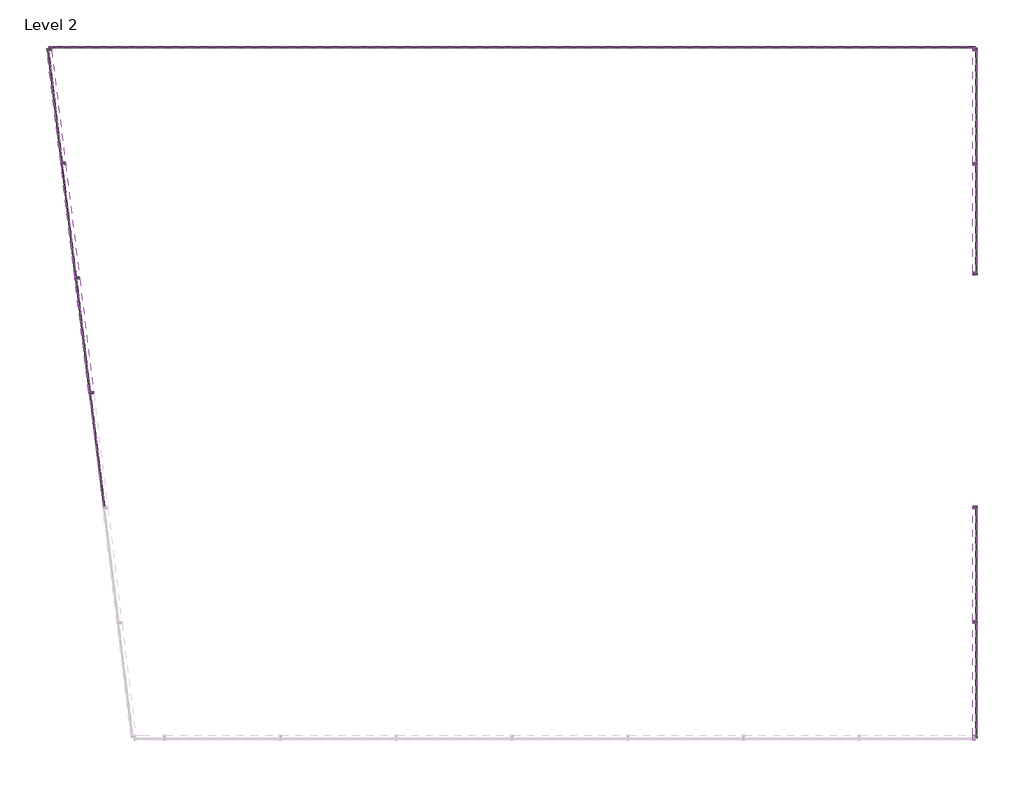
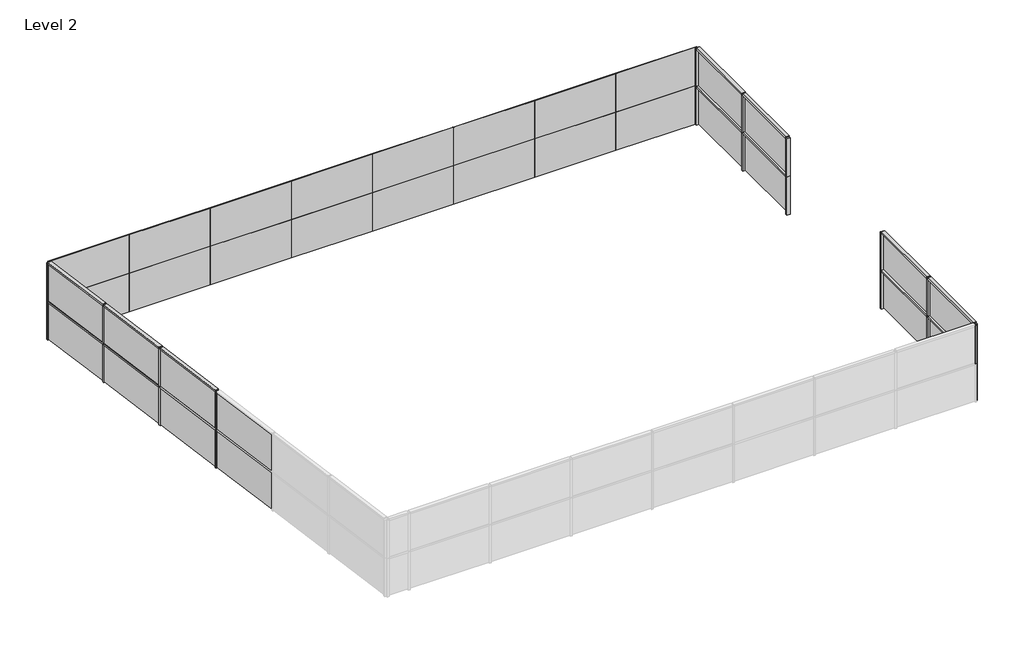
# One storey, part 2 of 2: 35 members, 32 plates.
"""IFC4 building model written with IfcOpenShell, lengths in millimetres."""

from ifc_helpers import new_model, si_unit, origin, place, context, project, spatial, transform, mapped, element, save
from components import member_19d0a4ec, member_8cef0660, member_82905deb, member_4491d118, member_46bdb8c2, system_panel_glazed_1e57f9bb, system_panel_glazed_e46d4b42, system_panel_glazed_2a6c68b7, system_panel_glazed_d483336f

model = new_model("IFC4")

# Units and contexts
model_context = context("Model", 3, world=origin())
ifc_project = project(units=[si_unit("LENGTHUNIT", "METRE", prefix="MILLI")], contexts=[model_context])

# Site, building, storey
site = spatial("IfcSite", under=ifc_project)
building = spatial("IfcBuilding", under=site)
storey = spatial("IfcBuildingStorey", under=building, Name="Level 2", Elevation=3048.0)

# Members
placement = place(None, origin())
member_shape = member_19d0a4ec(model_context)
element("IfcMember", 1, ObjectType="Rectangular Mullion : 2.5\" x 5\" rectangular", at=placement, inside=storey, context=model_context, shape_type="MappedRepresentation", body=[
    mapped(member_shape, transform((-10113.8959567, 8178.7803212, 4572.0), x_axis=(0.0, 0.0, 1.0), y_axis=(-0.9925461516413222, -0.12186934340514595, 0.0), z_axis=(0.12186934340514594, -0.9925461516413221, 0.0))),
])
element("IfcMember", 2, ObjectType="Rectangular Mullion : 2.5\" x 5\" rectangular", at=placement, inside=storey, context=model_context, shape_type="MappedRepresentation", body=[
    mapped(member_shape, transform((-10113.8959567, 8178.7803212, 6096.0), x_axis=(0.0, 0.0, 1.0), y_axis=(-0.9925461516413222, -0.12186934340514603, 0.0), z_axis=(0.12186934340514602, -0.9925461516413221, 0.0))),
])
element("IfcMember", 3, ObjectType="Rectangular Mullion : 2.5\" x 5\" rectangular", at=placement, inside=storey, context=model_context, shape_type="MappedRepresentation", body=[
    mapped(member_shape, transform((13902.5156363, 11109.0476508, 4572.0), x_axis=(0.0, 0.0, 1.0), y_axis=(1.0, 0.0, 0.0), z_axis=(0.0, 1.0, 0.0))),
])
element("IfcMember", 4, ObjectType="Rectangular Mullion : 2.5\" x 5\" rectangular", at=placement, inside=storey, context=model_context, shape_type="MappedRepresentation", body=[
    mapped(member_shape, transform((13902.5156363, 11109.0476508, 6096.0), x_axis=(0.0, 0.0, 1.0), y_axis=(1.0, 0.0, 0.0), z_axis=(0.0, 1.0, 0.0))),
])
element("IfcMember", 5, ObjectType="Rectangular Mullion : 2.5\" x 5\" rectangular", at=placement, inside=storey, context=model_context, shape_type="MappedRepresentation", body=[
    mapped(member_shape, transform((13902.5156363, -946.6363705, 4572.0), x_axis=(0.0, 0.0, 1.0), y_axis=(1.0, 0.0, 0.0), z_axis=(0.0, 1.0, 0.0))),
])
element("IfcMember", 6, ObjectType="Rectangular Mullion : 2.5\" x 5\" rectangular", at=placement, inside=storey, context=model_context, shape_type="MappedRepresentation", body=[
    mapped(member_shape, transform((13902.5156363, -3962.8863708, 4572.0), x_axis=(0.0, 0.0, 1.0), y_axis=(1.0, 0.0, 0.0), z_axis=(0.0, 1.0, 0.0))),
])
element("IfcMember", 7, ObjectType="Rectangular Mullion : 2.5\" x 5\" rectangular", at=placement, inside=storey, context=model_context, shape_type="MappedRepresentation", body=[
    mapped(member_shape, transform((13902.5156363, -946.6363705, 6096.0), x_axis=(0.0, 0.0, 1.0), y_axis=(1.0, 0.0, 0.0), z_axis=(0.0, 1.0, 0.0))),
])
element("IfcMember", 8, ObjectType="Rectangular Mullion : 2.5\" x 5\" rectangular", at=placement, inside=storey, context=model_context, shape_type="MappedRepresentation", body=[
    mapped(member_shape, transform((13902.5156363, -3962.8863708, 6096.0), x_axis=(0.0, 0.0, 1.0), y_axis=(1.0, 0.0, 0.0), z_axis=(0.0, 1.0, 0.0))),
])
member_2_shape = member_8cef0660(model_context)
element("IfcMember", 9, ObjectType="Rectangular Mullion : 2.5\" x 5\" rectangular", at=placement, inside=storey, context=model_context, shape_type="MappedRepresentation", body=[
    mapped(member_2_shape, transform((-9370.9804393, 2128.2189808, 4572.0), x_axis=(0.0, 0.0, 1.0), y_axis=(-0.9925461516413223, -0.12186934340514563, 0.0), z_axis=(0.12186934340514562, -0.9925461516413222, 0.0))),
])
element("IfcMember", 10, ObjectType="Rectangular Mullion : 2.5\" x 5\" rectangular", at=placement, inside=storey, context=model_context, shape_type="MappedRepresentation", body=[
    mapped(member_2_shape, transform((-9742.438198, 5153.499651, 4572.0), x_axis=(0.0, 0.0, 1.0), y_axis=(-0.9925461516413222, -0.12186934340514596, 0.0), z_axis=(0.12186934340514596, -0.9925461516413222, 0.0))),
])
element("IfcMember", 11, ObjectType="Rectangular Mullion : 2.5\" x 5\" rectangular", at=placement, inside=storey, context=model_context, shape_type="MappedRepresentation", body=[
    mapped(member_2_shape, transform((-9370.9804393, 2128.2189808, 6096.0), x_axis=(0.0, 0.0, 1.0), y_axis=(-0.9925461516413223, -0.12186934340514563, 0.0), z_axis=(0.12186934340514562, -0.9925461516413222, 0.0))),
])
element("IfcMember", 12, ObjectType="Rectangular Mullion : 2.5\" x 5\" rectangular", at=placement, inside=storey, context=model_context, shape_type="MappedRepresentation", body=[
    mapped(member_2_shape, transform((-9742.438198, 5153.499651, 6096.0), x_axis=(0.0, 0.0, 1.0), y_axis=(-0.9925461516413222, -0.12186934340514596, 0.0), z_axis=(0.12186934340514596, -0.9925461516413222, 0.0))),
])
member_3_shape = member_82905deb(model_context)
element("IfcMember", 13, ObjectType="Rectangular Mullion : 2.5\" x 5\" rectangular", at=placement, inside=storey, context=model_context, shape_type="MappedRepresentation", body=[
    mapped(member_3_shape, transform((-9367.1110876, 2096.7056405, 4572.0), x_axis=(-0.12186934340514591, 0.9925461516413222, 0.0), y_axis=(-0.9925461516413222, -0.12186934340514591, 0.0), z_axis=(0.0, 0.0, 1.0))),
])
element("IfcMember", 14, ObjectType="Rectangular Mullion : 2.5\" x 5\" rectangular", at=placement, inside=storey, context=model_context, shape_type="MappedRepresentation", body=[
    mapped(member_3_shape, transform((-9367.1110876, 2096.7056405, 6096.0), x_axis=(-0.12186934340514591, 0.9925461516413222, 0.0), y_axis=(-0.9925461516413222, -0.12186934340514591, 0.0), z_axis=(0.0, 0.0, 1.0))),
])
element("IfcMember", 15, ObjectType="Rectangular Mullion : 2.5\" x 5\" rectangular", at=placement, inside=storey, context=model_context, shape_type="MappedRepresentation", body=[
    mapped(member_3_shape, transform((-9738.5688463, 5121.9863107, 4572.0), x_axis=(-0.12186934340514591, 0.9925461516413222, 0.0), y_axis=(-0.9925461516413222, -0.12186934340514591, 0.0), z_axis=(0.0, 0.0, 1.0))),
])
element("IfcMember", 16, ObjectType="Rectangular Mullion : 2.5\" x 5\" rectangular", at=placement, inside=storey, context=model_context, shape_type="MappedRepresentation", body=[
    mapped(member_3_shape, transform((-9738.5688463, 5121.9863107, 6096.0), x_axis=(-0.12186934340514591, 0.9925461516413222, 0.0), y_axis=(-0.9925461516413222, -0.12186934340514591, 0.0), z_axis=(0.0, 0.0, 1.0))),
])
element("IfcMember", 17, ObjectType="Rectangular Mullion : 2.5\" x 5\" rectangular", at=placement, inside=storey, context=model_context, shape_type="MappedRepresentation", body=[
    mapped(member_3_shape, transform((-10110.026605, 8147.2669809, 4572.0), x_axis=(-0.12186934340514591, 0.9925461516413222, 0.0), y_axis=(-0.9925461516413222, -0.12186934340514591, 0.0), z_axis=(0.0, 0.0, 1.0))),
])
element("IfcMember", 18, ObjectType="Rectangular Mullion : 2.5\" x 5\" rectangular", at=placement, inside=storey, context=model_context, shape_type="MappedRepresentation", body=[
    mapped(member_3_shape, transform((-10110.026605, 8147.2669809, 6096.0), x_axis=(-0.12186934340514591, 0.9925461516413222, 0.0), y_axis=(-0.9925461516413222, -0.12186934340514591, 0.0), z_axis=(0.0, 0.0, 1.0))),
])
element("IfcMember", 19, ObjectType="Rectangular Mullion : 2.5\" x 5\" rectangular", at=placement, inside=storey, context=model_context, shape_type="MappedRepresentation", body=[
    mapped(member_3_shape, transform((13902.5156363, 8124.5476505, 4572.0), x_axis=(0.0, -1.0, 0.0), y_axis=(1.0, 0.0, 0.0), z_axis=(0.0, 0.0, 1.0))),
])
element("IfcMember", 20, ObjectType="Rectangular Mullion : 2.5\" x 5\" rectangular", at=placement, inside=storey, context=model_context, shape_type="MappedRepresentation", body=[
    mapped(member_3_shape, transform((13902.5156363, 8124.5476505, 6096.0), x_axis=(0.0, -1.0, 0.0), y_axis=(1.0, 0.0, 0.0), z_axis=(0.0, 0.0, 1.0))),
])
element("IfcMember", 21, ObjectType="Rectangular Mullion : 2.5\" x 5\" rectangular", at=placement, inside=storey, context=model_context, shape_type="MappedRepresentation", body=[
    mapped(member_3_shape, transform((13902.5156363, -3931.1363708, 4572.0), x_axis=(0.0, -1.0, 0.0), y_axis=(1.0, 0.0, 0.0), z_axis=(0.0, 0.0, 1.0))),
])
element("IfcMember", 22, ObjectType="Rectangular Mullion : 2.5\" x 5\" rectangular", at=placement, inside=storey, context=model_context, shape_type="MappedRepresentation", body=[
    mapped(member_3_shape, transform((13902.5156363, -3931.1363708, 6096.0), x_axis=(0.0, -1.0, 0.0), y_axis=(1.0, 0.0, 0.0), z_axis=(0.0, 0.0, 1.0))),
])
member_4_shape = member_4491d118(model_context)
element("IfcMember", 23, ObjectType="Rectangular Mullion : 2.5\" x 5\" rectangular", at=placement, inside=storey, context=model_context, shape_type="MappedRepresentation", body=[
    mapped(member_4_shape, transform((13902.5156363, -6979.1363705, 4572.0), x_axis=(1.0, 0.0, 0.0), y_axis=(0.0, -1.0, 0.0), z_axis=(0.0, 0.0, -1.0))),
])
element("IfcMember", 24, ObjectType="Rectangular Mullion : 2.5\" x 5\" rectangular", at=placement, inside=storey, context=model_context, shape_type="MappedRepresentation", body=[
    mapped(member_4_shape, transform((13902.5156363, 11172.5476508, 3048.0), x_axis=(0.0, 1.0, 0.0), y_axis=(1.0, 0.0, 0.0), z_axis=(0.0, 0.0, -1.0))),
])
element("IfcMember", 25, ObjectType="Rectangular Mullion : 2.5\" x 5\" rectangular", at=placement, inside=storey, context=model_context, shape_type="MappedRepresentation", body=[
    mapped(member_4_shape, transform((13902.5156363, 11172.5476508, 4572.0), x_axis=(0.0, 1.0, 0.0), y_axis=(1.0, 0.0, 0.0), z_axis=(0.0, 0.0, -1.0))),
])
element("IfcMember", 26, ObjectType="Rectangular Mullion : 2.5\" x 5\" rectangular", at=placement, inside=storey, context=model_context, shape_type="MappedRepresentation", body=[
    mapped(member_4_shape, transform((13902.5156363, -883.1363705, 3048.0), x_axis=(0.0, 1.0, 0.0), y_axis=(1.0, 0.0, 0.0), z_axis=(0.0, 0.0, -1.0))),
])
element("IfcMember", 27, ObjectType="Rectangular Mullion : 2.5\" x 5\" rectangular", at=placement, inside=storey, context=model_context, shape_type="MappedRepresentation", body=[
    mapped(member_4_shape, transform((13902.5156363, -883.1363705, 4572.0), x_axis=(0.0, 1.0, 0.0), y_axis=(1.0, 0.0, 0.0), z_axis=(0.0, 0.0, -1.0))),
])
element("IfcMember", 28, ObjectType="Rectangular Mullion : 2.5\" x 5\" rectangular", at=placement, inside=storey, context=model_context, shape_type="MappedRepresentation", body=[
    mapped(member_4_shape, transform((-10481.4843637, 11172.5476508, 4572.0), x_axis=(-0.12186934340514591, 0.9925461516413222, 0.0), y_axis=(-0.9925461516413222, -0.12186934340514591, 0.0), z_axis=(0.0, 0.0, 1.0))),
])
element("IfcMember", 29, ObjectType="Rectangular Mullion : 2.5\" x 5\" rectangular", at=placement, inside=storey, context=model_context, shape_type="MappedRepresentation", body=[
    mapped(member_4_shape, transform((-10481.4843637, 11172.5476508, 6096.0), x_axis=(-0.12186934340514591, 0.9925461516413222, 0.0), y_axis=(-0.9925461516413222, -0.12186934340514591, 0.0), z_axis=(0.0, 0.0, 1.0))),
])
element("IfcMember", 30, ObjectType="Rectangular Mullion : 2.5\" x 5\" rectangular", at=placement, inside=storey, context=model_context, shape_type="MappedRepresentation", body=[
    mapped(member_4_shape, transform((13902.5156363, 5212.8636295, 4572.0), x_axis=(0.0, -1.0, 0.0), y_axis=(1.0, 0.0, 0.0), z_axis=(0.0, 0.0, 1.0))),
])
element("IfcMember", 31, ObjectType="Rectangular Mullion : 2.5\" x 5\" rectangular", at=placement, inside=storey, context=model_context, shape_type="MappedRepresentation", body=[
    mapped(member_4_shape, transform((13902.5156363, 5212.8636295, 6096.0), x_axis=(0.0, -1.0, 0.0), y_axis=(1.0, 0.0, 0.0), z_axis=(0.0, 0.0, 1.0))),
])
element("IfcMember", 32, ObjectType="Rectangular Mullion : 2.5\" x 5\" rectangular", at=placement, inside=storey, context=model_context, shape_type="MappedRepresentation", body=[
    mapped(member_4_shape, transform((13902.5156363, -6979.1363705, 4572.0), x_axis=(0.0, -1.0, 0.0), y_axis=(1.0, 0.0, 0.0), z_axis=(0.0, 0.0, 1.0))),
])
element("IfcMember", 33, ObjectType="Rectangular Mullion : 2.5\" x 5\" rectangular", at=placement, inside=storey, context=model_context, shape_type="MappedRepresentation", body=[
    mapped(member_4_shape, transform((13902.5156363, -6979.1363705, 6096.0), x_axis=(0.0, -1.0, 0.0), y_axis=(1.0, 0.0, 0.0), z_axis=(0.0, 0.0, 1.0))),
])
member_5_shape = member_46bdb8c2(model_context)
element("IfcMember", 34, ObjectType="Rectangular Mullion : 2.5\" x 5\" rectangular", at=placement, inside=storey, context=model_context, shape_type="MappedRepresentation", body=[
    mapped(member_5_shape, transform((13902.5156363, 8092.7976505, 4572.0), x_axis=(0.0, 0.0, 1.0), y_axis=(1.0, 0.0, 0.0), z_axis=(0.0, 1.0, 0.0))),
])
element("IfcMember", 35, ObjectType="Rectangular Mullion : 2.5\" x 5\" rectangular", at=placement, inside=storey, context=model_context, shape_type="MappedRepresentation", body=[
    mapped(member_5_shape, transform((13902.5156363, 8092.7976505, 6096.0), x_axis=(0.0, 0.0, 1.0), y_axis=(1.0, 0.0, 0.0), z_axis=(0.0, 1.0, 0.0))),
])

# Plates
system_panel_glazed_shape = system_panel_glazed_1e57f9bb(model_context)
element("IfcPlate", 36, ObjectType="System Panel : Glazed", at=placement, inside=storey, context=model_context, shape_type="MappedRepresentation", body=[
    mapped(system_panel_glazed_shape, transform((-8957.4843636, 11172.5476508, 3048.0), x_axis=(1.0, 0.0, 0.0), y_axis=(0.0, 1.0, 0.0), z_axis=(0.0, 0.0, 1.0))),
])
element("IfcPlate", 37, ObjectType="System Panel : Glazed", at=placement, inside=storey, context=model_context, shape_type="MappedRepresentation", body=[
    mapped(system_panel_glazed_shape, transform((-5909.4843634, 11172.5476508, 3048.0), x_axis=(1.0, 0.0, 0.0), y_axis=(0.0, 1.0, 0.0), z_axis=(0.0, 0.0, 1.0))),
])
element("IfcPlate", 38, ObjectType="System Panel : Glazed", at=placement, inside=storey, context=model_context, shape_type="MappedRepresentation", body=[
    mapped(system_panel_glazed_shape, transform((-2861.4843634, 11172.5476508, 3048.0), x_axis=(1.0, 0.0, 0.0), y_axis=(0.0, 1.0, 0.0), z_axis=(0.0, 0.0, 1.0))),
])
element("IfcPlate", 39, ObjectType="System Panel : Glazed", at=placement, inside=storey, context=model_context, shape_type="MappedRepresentation", body=[
    mapped(system_panel_glazed_shape, transform((186.5156366, 11172.5476508, 3048.0), x_axis=(1.0, 0.0, 0.0), y_axis=(0.0, 1.0, 0.0), z_axis=(0.0, 0.0, 1.0))),
])
element("IfcPlate", 40, ObjectType="System Panel : Glazed", at=placement, inside=storey, context=model_context, shape_type="MappedRepresentation", body=[
    mapped(system_panel_glazed_shape, transform((3234.5156366, 11172.5476508, 3048.0), x_axis=(1.0, 0.0, 0.0), y_axis=(0.0, 1.0, 0.0), z_axis=(0.0, 0.0, 1.0))),
])
element("IfcPlate", 41, ObjectType="System Panel : Glazed", at=placement, inside=storey, context=model_context, shape_type="MappedRepresentation", body=[
    mapped(system_panel_glazed_shape, transform((6282.5156366, 11172.5476508, 3048.0), x_axis=(1.0, 0.0, 0.0), y_axis=(0.0, 1.0, 0.0), z_axis=(0.0, 0.0, 1.0))),
])
element("IfcPlate", 42, ObjectType="System Panel : Glazed", at=placement, inside=storey, context=model_context, shape_type="MappedRepresentation", body=[
    mapped(system_panel_glazed_shape, transform((9330.5156366, 11172.5476508, 3048.0), x_axis=(1.0, 0.0, 0.0), y_axis=(0.0, 1.0, 0.0), z_axis=(0.0, 0.0, 1.0))),
])
element("IfcPlate", 43, ObjectType="System Panel : Glazed", at=placement, inside=storey, context=model_context, shape_type="MappedRepresentation", body=[
    mapped(system_panel_glazed_shape, transform((12378.5156364, 11172.5476508, 3048.0), x_axis=(1.0, 0.0, 0.0), y_axis=(0.0, 1.0, 0.0), z_axis=(0.0, 0.0, 1.0))),
])
element("IfcPlate", 44, ObjectType="System Panel : Glazed", at=placement, inside=storey, context=model_context, shape_type="MappedRepresentation", body=[
    mapped(system_panel_glazed_shape, transform((-8957.4843636, 11172.5476508, 4572.0), x_axis=(1.0, 0.0, 0.0), y_axis=(0.0, 1.0, 0.0), z_axis=(0.0, 0.0, 1.0))),
])
element("IfcPlate", 45, ObjectType="System Panel : Glazed", at=placement, inside=storey, context=model_context, shape_type="MappedRepresentation", body=[
    mapped(system_panel_glazed_shape, transform((-5909.4843634, 11172.5476508, 4572.0), x_axis=(1.0, 0.0, 0.0), y_axis=(0.0, 1.0, 0.0), z_axis=(0.0, 0.0, 1.0))),
])
element("IfcPlate", 46, ObjectType="System Panel : Glazed", at=placement, inside=storey, context=model_context, shape_type="MappedRepresentation", body=[
    mapped(system_panel_glazed_shape, transform((-2861.4843634, 11172.5476508, 4572.0), x_axis=(1.0, 0.0, 0.0), y_axis=(0.0, 1.0, 0.0), z_axis=(0.0, 0.0, 1.0))),
])
element("IfcPlate", 47, ObjectType="System Panel : Glazed", at=placement, inside=storey, context=model_context, shape_type="MappedRepresentation", body=[
    mapped(system_panel_glazed_shape, transform((186.5156366, 11172.5476508, 4572.0), x_axis=(1.0, 0.0, 0.0), y_axis=(0.0, 1.0, 0.0), z_axis=(0.0, 0.0, 1.0))),
])
element("IfcPlate", 48, ObjectType="System Panel : Glazed", at=placement, inside=storey, context=model_context, shape_type="MappedRepresentation", body=[
    mapped(system_panel_glazed_shape, transform((3234.5156366, 11172.5476508, 4572.0), x_axis=(1.0, 0.0, 0.0), y_axis=(0.0, 1.0, 0.0), z_axis=(0.0, 0.0, 1.0))),
])
element("IfcPlate", 49, ObjectType="System Panel : Glazed", at=placement, inside=storey, context=model_context, shape_type="MappedRepresentation", body=[
    mapped(system_panel_glazed_shape, transform((6282.5156366, 11172.5476508, 4572.0), x_axis=(1.0, 0.0, 0.0), y_axis=(0.0, 1.0, 0.0), z_axis=(0.0, 0.0, 1.0))),
])
element("IfcPlate", 50, ObjectType="System Panel : Glazed", at=placement, inside=storey, context=model_context, shape_type="MappedRepresentation", body=[
    mapped(system_panel_glazed_shape, transform((9330.5156366, 11172.5476508, 4572.0), x_axis=(1.0, 0.0, 0.0), y_axis=(0.0, 1.0, 0.0), z_axis=(0.0, 0.0, 1.0))),
])
element("IfcPlate", 51, ObjectType="System Panel : Glazed", at=placement, inside=storey, context=model_context, shape_type="MappedRepresentation", body=[
    mapped(system_panel_glazed_shape, transform((12378.5156364, 11172.5476508, 4572.0), x_axis=(1.0, 0.0, 0.0), y_axis=(0.0, 1.0, 0.0), z_axis=(0.0, 0.0, 1.0))),
])
system_panel_glazed_2_shape = system_panel_glazed_e46d4b42(model_context)
element("IfcPlate", 52, ObjectType="System Panel : Glazed", at=placement, inside=storey, context=model_context, shape_type="MappedRepresentation", body=[
    mapped(system_panel_glazed_2_shape, transform((-10293.8208085, 9644.1506457, 3079.75), x_axis=(-0.12186934340514591, 0.9925461516413222, 0.0), y_axis=(-0.9925461516413222, -0.12186934340514591, 0.0), z_axis=(0.0, 0.0, 1.0))),
])
element("IfcPlate", 53, ObjectType="System Panel : Glazed", at=placement, inside=storey, context=model_context, shape_type="MappedRepresentation", body=[
    mapped(system_panel_glazed_2_shape, transform((-10293.8208085, 9644.1506457, 4603.75), x_axis=(-0.12186934340514591, 0.9925461516413222, 0.0), y_axis=(-0.9925461516413222, -0.12186934340514591, 0.0), z_axis=(0.0, 0.0, 1.0))),
])
element("IfcPlate", 54, ObjectType="System Panel : Glazed", at=placement, inside=storey, context=model_context, shape_type="MappedRepresentation", body=[
    mapped(system_panel_glazed_2_shape, transform((13902.5156363, -2423.0113706, 3079.75), x_axis=(0.0, -1.0, 0.0), y_axis=(1.0, 0.0, 0.0), z_axis=(0.0, 0.0, 1.0))),
])
element("IfcPlate", 55, ObjectType="System Panel : Glazed", at=placement, inside=storey, context=model_context, shape_type="MappedRepresentation", body=[
    mapped(system_panel_glazed_2_shape, transform((13902.5156363, -5439.2613706, 3079.75), x_axis=(0.0, -1.0, 0.0), y_axis=(1.0, 0.0, 0.0), z_axis=(0.0, 0.0, 1.0))),
])
element("IfcPlate", 56, ObjectType="System Panel : Glazed", at=placement, inside=storey, context=model_context, shape_type="MappedRepresentation", body=[
    mapped(system_panel_glazed_2_shape, transform((13902.5156363, -2423.0113706, 4603.75), x_axis=(0.0, -1.0, 0.0), y_axis=(1.0, 0.0, 0.0), z_axis=(0.0, 0.0, 1.0))),
])
element("IfcPlate", 57, ObjectType="System Panel : Glazed", at=placement, inside=storey, context=model_context, shape_type="MappedRepresentation", body=[
    mapped(system_panel_glazed_2_shape, transform((13902.5156363, -5439.2613706, 4603.75), x_axis=(0.0, -1.0, 0.0), y_axis=(1.0, 0.0, 0.0), z_axis=(0.0, 0.0, 1.0))),
])
element("IfcPlate", 58, ObjectType="System Panel : Glazed", at=placement, inside=storey, context=model_context, shape_type="MappedRepresentation", body=[
    mapped(system_panel_glazed_2_shape, transform((13902.5156363, 9632.6726506, 3079.75), x_axis=(0.0, -1.0, 0.0), y_axis=(1.0, 0.0, 0.0), z_axis=(0.0, 0.0, 1.0))),
])
element("IfcPlate", 59, ObjectType="System Panel : Glazed", at=placement, inside=storey, context=model_context, shape_type="MappedRepresentation", body=[
    mapped(system_panel_glazed_2_shape, transform((13902.5156363, 9632.6726506, 4603.75), x_axis=(0.0, -1.0, 0.0), y_axis=(1.0, 0.0, 0.0), z_axis=(0.0, 0.0, 1.0))),
])
system_panel_glazed_3_shape = system_panel_glazed_2a6c68b7(model_context)
element("IfcPlate", 60, ObjectType="System Panel : Glazed", at=placement, inside=storey, context=model_context, shape_type="MappedRepresentation", body=[
    mapped(system_panel_glazed_3_shape, transform((-9181.3822083, 584.0653054, 3079.75), x_axis=(-0.12186934340514591, 0.9925461516413222, 0.0), y_axis=(-0.9925461516413222, -0.12186934340514591, 0.0), z_axis=(0.0, 0.0, 1.0))),
])
element("IfcPlate", 61, ObjectType="System Panel : Glazed", at=placement, inside=storey, context=model_context, shape_type="MappedRepresentation", body=[
    mapped(system_panel_glazed_3_shape, transform((-9552.839967, 3609.3459756, 3079.75), x_axis=(-0.12186934340514591, 0.9925461516413222, 0.0), y_axis=(-0.9925461516413222, -0.12186934340514591, 0.0), z_axis=(0.0, 0.0, 1.0))),
])
element("IfcPlate", 62, ObjectType="System Panel : Glazed", at=placement, inside=storey, context=model_context, shape_type="MappedRepresentation", body=[
    mapped(system_panel_glazed_3_shape, transform((-9924.2977257, 6634.6266458, 3079.75), x_axis=(-0.12186934340514591, 0.9925461516413222, 0.0), y_axis=(-0.9925461516413222, -0.12186934340514591, 0.0), z_axis=(0.0, 0.0, 1.0))),
])
element("IfcPlate", 63, ObjectType="System Panel : Glazed", at=placement, inside=storey, context=model_context, shape_type="MappedRepresentation", body=[
    mapped(system_panel_glazed_3_shape, transform((-9181.3822083, 584.0653054, 4603.75), x_axis=(-0.12186934340514591, 0.9925461516413222, 0.0), y_axis=(-0.9925461516413222, -0.12186934340514591, 0.0), z_axis=(0.0, 0.0, 1.0))),
])
element("IfcPlate", 64, ObjectType="System Panel : Glazed", at=placement, inside=storey, context=model_context, shape_type="MappedRepresentation", body=[
    mapped(system_panel_glazed_3_shape, transform((-9552.839967, 3609.3459756, 4603.75), x_axis=(-0.12186934340514591, 0.9925461516413222, 0.0), y_axis=(-0.9925461516413222, -0.12186934340514591, 0.0), z_axis=(0.0, 0.0, 1.0))),
])
element("IfcPlate", 65, ObjectType="System Panel : Glazed", at=placement, inside=storey, context=model_context, shape_type="MappedRepresentation", body=[
    mapped(system_panel_glazed_3_shape, transform((-9924.2977257, 6634.6266458, 4603.75), x_axis=(-0.12186934340514591, 0.9925461516413222, 0.0), y_axis=(-0.9925461516413222, -0.12186934340514591, 0.0), z_axis=(0.0, 0.0, 1.0))),
])
system_panel_glazed_4_shape = system_panel_glazed_d483336f(model_context)
element("IfcPlate", 66, ObjectType="System Panel : Glazed", at=placement, inside=storey, context=model_context, shape_type="MappedRepresentation", body=[
    mapped(system_panel_glazed_4_shape, transform((13902.5156363, 6684.58064, 3079.75), x_axis=(0.0, -1.0, 0.0), y_axis=(1.0, 0.0, 0.0), z_axis=(0.0, 0.0, 1.0))),
])
element("IfcPlate", 67, ObjectType="System Panel : Glazed", at=placement, inside=storey, context=model_context, shape_type="MappedRepresentation", body=[
    mapped(system_panel_glazed_4_shape, transform((13902.5156363, 6684.58064, 4603.75), x_axis=(0.0, -1.0, 0.0), y_axis=(1.0, 0.0, 0.0), z_axis=(0.0, 0.0, 1.0))),
])

save(model, "model.ifc")

# Revit data of these elements
# Type "Rectangular Mullion : 2.5\" x 5\" rectangular"
#   built-in parameter 1007304 = 0.416667 (stored number, unit not read)
#   built-in parameter 1007301 = 0.104167 (stored number, unit not read)
#   built-in parameter 1007300 = 0.104167 (stored number, unit not read)
# Type "System Panel : Glazed"
#   Construction Type Id = "GSP4R"
#   Analytic Construction = "1/8 in Pilkington single glazing"
#   Visual Light Transmittance = 0.9
#   Solar Heat Gain Coefficient = 0.86
#   Heat Transfer Coefficient (U) = 1.18115 BTU/(h·ft²·°F)
#   Define Thermal Properties by = 1
# Elements 1, 2, 3, 4, 5, 6, 7, 8, 9, 10, 11, 12, 13, 14, 15, 16, 17, 18, 19, 20, 21, 22, 23, 24, 25, 26, 27, 28, 29, 30, 31, 32, 33, 34, 35 (IfcMember, "Rectangular Mullion : 2.5\" x 5\" rectangular")
#   Phase Created = New Construction
#   Materials on its faces: "Aluminum"
# Elements 36, 37, 38, 39, 40, 41, 42, 43, 44, 45, 46, 47, 48, 49, 50, 51, 52, 53, 54, 55, 56, 57, 58, 59, 60, 61, 62, 63, 64, 65, 66, 67 (IfcPlate, "System Panel : Glazed")
#   Phase Created = New Construction
#   Materials on its faces: "Glass"
# Materials
#   "Aluminum": class "Metal", colour RGB 247 247 247, transparency 0, Description = "Aluminum 6061", Cost = 0
#   "Glass": class "Glass", colour RGB 0 128 192, transparency 0.75, Description = "Soda Lime Glass", Cost = 0
